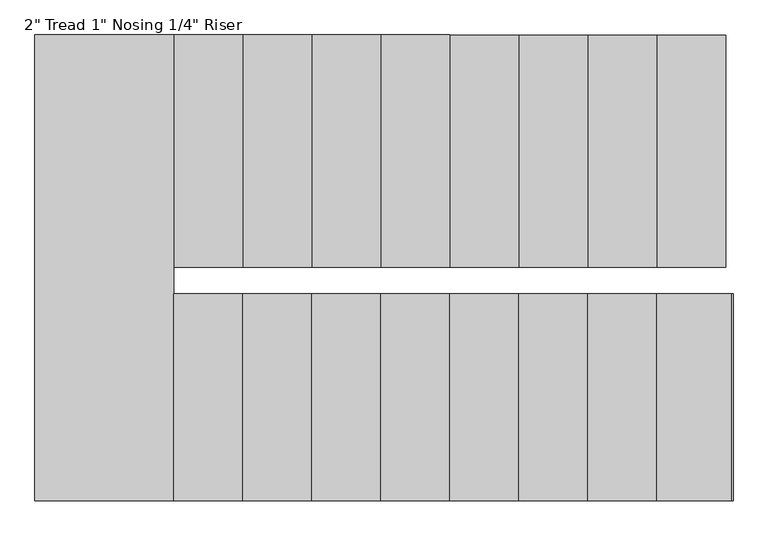
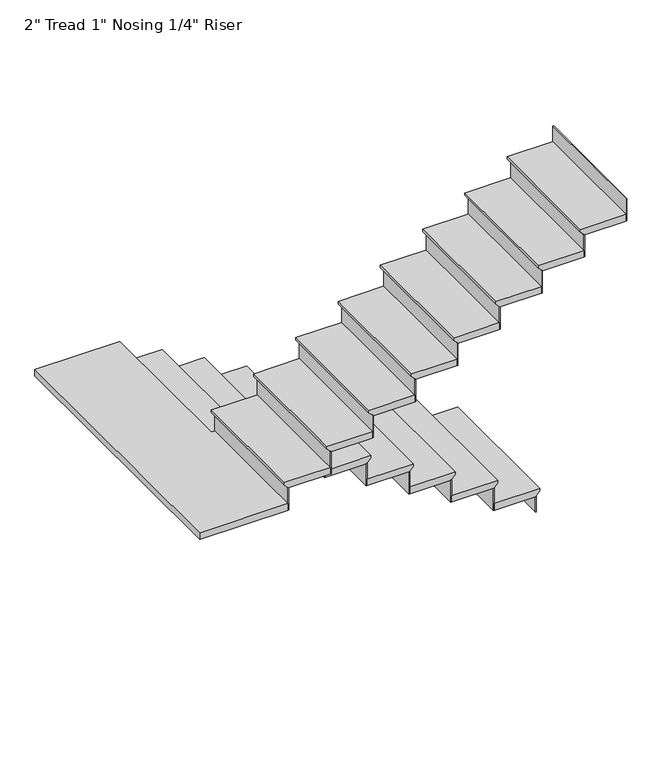
"""IFC4 building model written with IfcOpenShell, lengths in millimetres: stair flight geometry."""

from ifc_helpers import new_model, si_unit, origin, place, context, project, spatial, faceted_brep, source, transform, mapped, element, save


def stair_flight_67f7f0a7(model_context):
    return source(origin(), model_context, "Body", "Brep", [
        faceted_brep([(4295.1355783, 9969.5, 6246.2833333), (4295.1355783, 9969.5, 6265.3333333), (4295.1355783, 8944.6068332, 6265.3333333), (4295.1355783, 8944.6068332, 6246.2833333), (4269.7355783, 9969.5, 6220.8833333), (4269.7355783, 8944.6068332, 6220.8833333), (3964.9355783, 9969.5, 6265.3333333), (3964.9355783, 8944.6068332, 6265.3333333), (4269.7355783, 8944.6068332, 6214.5333333), (3964.9355783, 8944.6068332, 6214.5333333), (3964.9355783, 9969.5, 6214.5333333), (4269.7355783, 9969.5, 6214.5333333)], [[[0, 1, 2, 3]], [[4, 0, 3, 5]], [[2, 1, 6, 7]], [[8, 9, 10, 11]], [[2, 7, 9, 8, 5, 3]], [[8, 11, 4, 5]], [[6, 1, 0, 4, 11, 10]], [[7, 6, 10, 9]]]),
        faceted_brep([(4269.7355783, 9969.5, 6214.5333333), (4269.7355783, 9969.5, 6096.0), (4263.3855783, 9969.5, 6096.0), (4263.3855783, 9969.5, 6214.5333333), (4269.7355783, 8944.6068332, 6214.5333333), (4263.3855783, 8944.6068332, 6214.5333333), (4263.3855783, 8944.6068332, 6096.0), (4269.7355783, 8944.6068332, 6096.0)], [[[0, 1, 2, 3]], [[4, 5, 6, 7]], [[1, 0, 4, 7]], [[2, 1, 7, 6]], [[3, 2, 6, 5]], [[0, 3, 5, 4]]]),
        faceted_brep([(3964.9355783, 9969.5, 6383.8666667), (3964.9355783, 9969.5, 6214.5333333), (3958.5855783, 9969.5, 6214.5333333), (3958.5855783, 9969.5, 6383.8666667), (3964.9355783, 8944.6068332, 6383.8666667), (3958.5855783, 8944.6068332, 6383.8666667), (3958.5855783, 8944.6068332, 6214.5333333), (3964.9355783, 8944.6068332, 6214.5333333)], [[[0, 1, 2, 3]], [[4, 5, 6, 7]], [[1, 0, 4, 7]], [[2, 1, 7, 6]], [[3, 2, 6, 5]], [[0, 3, 5, 4]]]),
        faceted_brep([(3990.3355783, 8944.6068332, 6434.6666667), (3990.3355783, 9969.5, 6434.6666667), (3660.1355783, 9969.5, 6434.6666667), (3660.1355783, 8944.6068332, 6434.6666667), (3964.9355783, 8944.6068332, 6383.8666667), (3660.1355783, 8944.6068332, 6383.8666667), (3660.1355783, 9969.5, 6383.8666667), (3964.9355783, 9969.5, 6383.8666667), (3964.9355783, 8944.6068332, 6390.2166667), (3990.3355783, 8944.6068332, 6415.6166667), (3964.9355783, 9969.5, 6390.2166667), (3990.3355783, 9969.5, 6415.6166667)], [[[0, 1, 2, 3]], [[4, 5, 6, 7]], [[0, 3, 5, 4, 8, 9]], [[4, 7, 10, 8]], [[2, 1, 11, 10, 7, 6]], [[3, 2, 6, 5]], [[11, 1, 0, 9]], [[10, 11, 9, 8]]]),
        faceted_brep([(3660.1355783, 9969.5, 6553.2), (3660.1355783, 9969.5, 6383.8666667), (3653.7855783, 9969.5, 6383.8666667), (3653.7855783, 9969.5, 6553.2), (3660.1355783, 8944.6068332, 6553.2), (3653.7855783, 8944.6068332, 6553.2), (3653.7855783, 8944.6068332, 6383.8666667), (3660.1355783, 8944.6068332, 6383.8666667)], [[[0, 1, 2, 3]], [[4, 5, 6, 7]], [[1, 0, 4, 7]], [[2, 1, 7, 6]], [[3, 2, 6, 5]], [[0, 3, 5, 4]]]),
        faceted_brep([(3685.5355783, 8944.6068332, 6604.0), (3685.5355783, 9969.5, 6604.0), (3355.3355783, 9969.5, 6604.0), (3355.3355783, 8944.6068332, 6604.0), (3660.1355783, 8944.6068332, 6553.2), (3355.3355783, 8944.6068332, 6553.2), (3355.3355783, 9969.5, 6553.2), (3660.1355783, 9969.5, 6553.2), (3660.1355783, 8944.6068332, 6559.55), (3685.5355783, 8944.6068332, 6584.95), (3660.1355783, 9969.5, 6559.55), (3685.5355783, 9969.5, 6584.95)], [[[0, 1, 2, 3]], [[4, 5, 6, 7]], [[0, 3, 5, 4, 8, 9]], [[4, 7, 10, 8]], [[2, 1, 11, 10, 7, 6]], [[3, 2, 6, 5]], [[11, 1, 0, 9]], [[10, 11, 9, 8]]]),
        faceted_brep([(3355.3355783, 9969.5, 6722.5333333), (3355.3355783, 9969.5, 6553.2), (3348.9855783, 9969.5, 6553.2), (3348.9855783, 9969.5, 6722.5333333), (3355.3355783, 8944.6068332, 6722.5333333), (3348.9855783, 8944.6068332, 6722.5333333), (3348.9855783, 8944.6068332, 6553.2), (3355.3355783, 8944.6068332, 6553.2)], [[[0, 1, 2, 3]], [[4, 5, 6, 7]], [[1, 0, 4, 7]], [[2, 1, 7, 6]], [[3, 2, 6, 5]], [[0, 3, 5, 4]]]),
        faceted_brep([(3380.7355783, 8944.6068332, 6773.3333333), (3380.7355783, 9969.5, 6773.3333333), (3050.5355783, 9969.5, 6773.3333333), (3050.5355783, 8944.6068332, 6773.3333333), (3355.3355783, 8944.6068332, 6722.5333333), (3050.5355783, 8944.6068332, 6722.5333333), (3050.5355783, 9969.5, 6722.5333333), (3355.3355783, 9969.5, 6722.5333333), (3355.3355783, 8944.6068332, 6728.8833333), (3380.7355783, 8944.6068332, 6754.2833333), (3355.3355783, 9969.5, 6728.8833333), (3380.7355783, 9969.5, 6754.2833333)], [[[0, 1, 2, 3]], [[4, 5, 6, 7]], [[0, 3, 5, 4, 8, 9]], [[4, 7, 10, 8]], [[2, 1, 11, 10, 7, 6]], [[3, 2, 6, 5]], [[11, 1, 0, 9]], [[10, 11, 9, 8]]]),
        faceted_brep([(3050.5355783, 9969.5, 6891.8666667), (3050.5355783, 9969.5, 6722.5333333), (3044.1855783, 9969.5, 6722.5333333), (3044.1855783, 9969.5, 6891.8666667), (3050.5355783, 8944.6068332, 6891.8666667), (3044.1855783, 8944.6068332, 6891.8666667), (3044.1855783, 8944.6068332, 6722.5333333), (3050.5355783, 8944.6068332, 6722.5333333)], [[[0, 1, 2, 3]], [[4, 5, 6, 7]], [[1, 0, 4, 7]], [[2, 1, 7, 6]], [[3, 2, 6, 5]], [[0, 3, 5, 4]]]),
        faceted_brep([(3075.9355783, 8944.6068332, 6942.6666667), (3075.9355783, 9969.5, 6942.6666667), (2745.7355783, 9969.5, 6942.6666667), (2745.7355783, 8944.6068332, 6942.6666667), (3050.5355783, 8944.6068332, 6891.8666667), (2745.7355783, 8944.6068332, 6891.8666667), (2745.7355783, 9969.5, 6891.8666667), (3050.5355783, 9969.5, 6891.8666667), (3050.5355783, 8944.6068332, 6898.2166667), (3075.9355783, 8944.6068332, 6923.6166667), (3050.5355783, 9969.5, 6898.2166667), (3075.9355783, 9969.5, 6923.6166667)], [[[0, 1, 2, 3]], [[4, 5, 6, 7]], [[0, 3, 5, 4, 8, 9]], [[4, 7, 10, 8]], [[2, 1, 11, 10, 7, 6]], [[3, 2, 6, 5]], [[11, 1, 0, 9]], [[10, 11, 9, 8]]]),
        faceted_brep([(2745.7355783, 9969.5, 7061.2), (2745.7355783, 9969.5, 6891.8666667), (2739.3855783, 9969.5, 6891.8666667), (2739.3855783, 9969.5, 7061.2), (2745.7355783, 8944.6068332, 7061.2), (2739.3855783, 8944.6068332, 7061.2), (2739.3855783, 8944.6068332, 6891.8666667), (2745.7355783, 8944.6068332, 6891.8666667)], [[[0, 1, 2, 3]], [[4, 5, 6, 7]], [[1, 0, 4, 7]], [[2, 1, 7, 6]], [[3, 2, 6, 5]], [[0, 3, 5, 4]]]),
        faceted_brep([(2771.1355783, 8944.6068332, 7112.0), (2771.1355783, 9969.5, 7112.0), (2440.9355783, 9969.5, 7112.0), (2440.9355783, 8944.6068332, 7112.0), (2745.7355783, 8944.6068332, 7061.2), (2440.9355783, 8944.6068332, 7061.2), (2440.9355783, 9969.5, 7061.2), (2745.7355783, 9969.5, 7061.2), (2745.7355783, 8944.6068332, 7067.55), (2771.1355783, 8944.6068332, 7092.95), (2745.7355783, 9969.5, 7067.55), (2771.1355783, 9969.5, 7092.95)], [[[0, 1, 2, 3]], [[4, 5, 6, 7]], [[0, 3, 5, 4, 8, 9]], [[4, 7, 10, 8]], [[2, 1, 11, 10, 7, 6]], [[3, 2, 6, 5]], [[11, 1, 0, 9]], [[10, 11, 9, 8]]]),
        faceted_brep([(2440.9355783, 9969.5, 7230.5333333), (2440.9355783, 9969.5, 7061.2), (2434.5855783, 9969.5, 7061.2), (2434.5855783, 9969.5, 7230.5333333), (2440.9355783, 8944.6068332, 7230.5333333), (2434.5855783, 8944.6068332, 7230.5333333), (2434.5855783, 8944.6068332, 7061.2), (2440.9355783, 8944.6068332, 7061.2)], [[[0, 1, 2, 3]], [[4, 5, 6, 7]], [[1, 0, 4, 7]], [[2, 1, 7, 6]], [[3, 2, 6, 5]], [[0, 3, 5, 4]]]),
        faceted_brep([(2466.3355783, 8944.6068332, 7281.3333333), (2466.3355783, 9969.5, 7281.3333333), (2136.1355783, 9969.5, 7281.3333333), (2136.1355783, 8944.6068332, 7281.3333333), (2440.9355783, 8944.6068332, 7230.5333333), (2136.1355783, 8944.6068332, 7230.5333333), (2136.1355783, 9969.5, 7230.5333333), (2440.9355783, 9969.5, 7230.5333333), (2440.9355783, 8944.6068332, 7236.8833333), (2466.3355783, 8944.6068332, 7262.2833333), (2440.9355783, 9969.5, 7236.8833333), (2466.3355783, 9969.5, 7262.2833333)], [[[0, 1, 2, 3]], [[4, 5, 6, 7]], [[0, 3, 5, 4, 8, 9]], [[4, 7, 10, 8]], [[2, 1, 11, 10, 7, 6]], [[3, 2, 6, 5]], [[11, 1, 0, 9]], [[10, 11, 9, 8]]]),
        faceted_brep([(2136.1355783, 9969.5, 7399.8666667), (2136.1355783, 9969.5, 7230.5333333), (2129.7855783, 9969.5, 7230.5333333), (2129.7855783, 9969.5, 7399.8666667), (2136.1355783, 8944.6068332, 7399.8666667), (2129.7855783, 8944.6068332, 7399.8666667), (2129.7855783, 8944.6068332, 7230.5333333), (2136.1355783, 8944.6068332, 7230.5333333)], [[[0, 1, 2, 3]], [[4, 5, 6, 7]], [[1, 0, 4, 7]], [[2, 1, 7, 6]], [[3, 2, 6, 5]], [[0, 3, 5, 4]]]),
        faceted_brep([(2161.5355783, 8944.6068332, 7450.6666667), (2161.5355783, 9969.5, 7450.6666667), (1831.3355783, 9969.5, 7450.6666667), (1831.3355783, 8944.6068332, 7450.6666667), (2136.1355783, 8944.6068332, 7399.8666667), (1831.3355783, 8944.6068332, 7399.8666667), (1831.3355783, 9969.5, 7399.8666667), (2136.1355783, 9969.5, 7399.8666667), (2136.1355783, 8944.6068332, 7406.2166667), (2161.5355783, 8944.6068332, 7431.6166667), (2136.1355783, 9969.5, 7406.2166667), (2161.5355783, 9969.5, 7431.6166667)], [[[0, 1, 2, 3]], [[4, 5, 6, 7]], [[0, 3, 5, 4, 8, 9]], [[4, 7, 10, 8]], [[2, 1, 11, 10, 7, 6]], [[3, 2, 6, 5]], [[11, 1, 0, 9]], [[10, 11, 9, 8]]]),
        faceted_brep([(1831.3355783, 9969.5, 7569.2), (1831.3355783, 9969.5, 7399.8666667), (1824.9855783, 9969.5, 7399.8666667), (1824.9855783, 9969.5, 7569.2), (1831.3355783, 8944.6068332, 7569.2), (1824.9855783, 8944.6068332, 7569.2), (1824.9855783, 8944.6068332, 7399.8666667), (1831.3355783, 8944.6068332, 7399.8666667)], [[[0, 1, 2, 3]], [[4, 5, 6, 7]], [[1, 0, 4, 7]], [[2, 1, 7, 6]], [[3, 2, 6, 5]], [[0, 3, 5, 4]]]),
        faceted_brep([(1882.1355783, 8826.5, 7620.0), (1856.7355783, 8826.5, 7620.0), (1856.7355783, 9969.5, 7620.0), (1244.6, 9969.5, 7620.0), (1244.6, 7912.1, 7620.0), (1882.1355783, 7912.1, 7620.0), (1856.7355783, 8826.5, 7569.2), (1882.1355783, 8826.5, 7569.2), (1882.1355783, 7912.1, 7569.2), (1244.6, 7912.1, 7569.2), (1244.6, 9969.5, 7569.2), (1831.3355783, 9969.5, 7569.2), (1831.3355783, 8944.6068332, 7569.2), (1856.7355783, 8944.6068332, 7569.2), (1856.7355783, 8944.6068332, 7600.95), (1856.7355783, 9969.5, 7600.95), (1831.3355783, 8944.6068332, 7575.55), (1831.3355783, 9969.5, 7575.55)], [[[0, 1, 2, 3, 4, 5]], [[6, 7, 8, 9, 10, 11, 12, 13]], [[1, 0, 7, 6]], [[2, 1, 6, 13, 14, 15]], [[13, 12, 16, 14]], [[12, 11, 17, 16]], [[3, 2, 15, 17, 11, 10]], [[4, 3, 10, 9]], [[5, 4, 9, 8]], [[0, 5, 8, 7]], [[17, 15, 14, 16]]]),
        faceted_brep([(1882.1355783, 7912.1, 7738.5333333), (1882.1355783, 7912.1, 7569.2), (1888.4855783, 7912.1, 7569.2), (1888.4855783, 7912.1, 7738.5333333), (1882.1355783, 8826.5, 7738.5333333), (1888.4855783, 8826.5, 7738.5333333), (1888.4855783, 8826.5, 7569.2), (1882.1355783, 8826.5, 7569.2)], [[[0, 1, 2, 3]], [[4, 5, 6, 7]], [[1, 0, 4, 7]], [[2, 1, 7, 6]], [[3, 2, 6, 5]], [[0, 3, 5, 4]]]),
        faceted_brep([(1856.7355783, 8826.5, 7789.3333333), (1856.7355783, 7912.1, 7789.3333333), (2186.9355783, 7912.1, 7789.3333333), (2186.9355783, 8826.5, 7789.3333333), (1882.1355783, 8826.5, 7738.5333333), (2186.9355783, 8826.5, 7738.5333333), (2186.9355783, 7912.1, 7738.5333333), (1882.1355783, 7912.1, 7738.5333333), (1882.1355783, 8826.5, 7744.8833333), (1856.7355783, 8826.5, 7770.2833333), (1882.1355783, 7912.1, 7744.8833333), (1856.7355783, 7912.1, 7770.2833333)], [[[0, 1, 2, 3]], [[4, 5, 6, 7]], [[0, 3, 5, 4, 8, 9]], [[4, 7, 10, 8]], [[2, 1, 11, 10, 7, 6]], [[3, 2, 6, 5]], [[11, 1, 0, 9]], [[10, 11, 9, 8]]]),
        faceted_brep([(2186.9355783, 7912.1, 7907.8666667), (2186.9355783, 7912.1, 7738.5333333), (2193.2855783, 7912.1, 7738.5333333), (2193.2855783, 7912.1, 7907.8666667), (2186.9355783, 8826.5, 7907.8666667), (2193.2855783, 8826.5, 7907.8666667), (2193.2855783, 8826.5, 7738.5333333), (2186.9355783, 8826.5, 7738.5333333)], [[[0, 1, 2, 3]], [[4, 5, 6, 7]], [[1, 0, 4, 7]], [[2, 1, 7, 6]], [[3, 2, 6, 5]], [[0, 3, 5, 4]]]),
        faceted_brep([(2161.5355783, 8826.5, 7958.6666667), (2161.5355783, 7912.1, 7958.6666667), (2491.7355783, 7912.1, 7958.6666667), (2491.7355783, 8826.5, 7958.6666667), (2186.9355783, 8826.5, 7907.8666667), (2491.7355783, 8826.5, 7907.8666667), (2491.7355783, 7912.1, 7907.8666667), (2186.9355783, 7912.1, 7907.8666667), (2186.9355783, 8826.5, 7914.2166667), (2161.5355783, 8826.5, 7939.6166667), (2186.9355783, 7912.1, 7914.2166667), (2161.5355783, 7912.1, 7939.6166667)], [[[0, 1, 2, 3]], [[4, 5, 6, 7]], [[0, 3, 5, 4, 8, 9]], [[4, 7, 10, 8]], [[2, 1, 11, 10, 7, 6]], [[3, 2, 6, 5]], [[11, 1, 0, 9]], [[10, 11, 9, 8]]]),
        faceted_brep([(2491.7355783, 7912.1, 8077.2), (2491.7355783, 7912.1, 7907.8666667), (2498.0855783, 7912.1, 7907.8666667), (2498.0855783, 7912.1, 8077.2), (2491.7355783, 8826.5, 8077.2), (2498.0855783, 8826.5, 8077.2), (2498.0855783, 8826.5, 7907.8666667), (2491.7355783, 8826.5, 7907.8666667)], [[[0, 1, 2, 3]], [[4, 5, 6, 7]], [[1, 0, 4, 7]], [[2, 1, 7, 6]], [[3, 2, 6, 5]], [[0, 3, 5, 4]]]),
        faceted_brep([(2466.3355783, 8826.5, 8128.0), (2466.3355783, 7912.1, 8128.0), (2796.5355783, 7912.1, 8128.0), (2796.5355783, 8826.5, 8128.0), (2491.7355783, 8826.5, 8077.2), (2796.5355783, 8826.5, 8077.2), (2796.5355783, 7912.1, 8077.2), (2491.7355783, 7912.1, 8077.2), (2491.7355783, 8826.5, 8083.55), (2466.3355783, 8826.5, 8108.95), (2491.7355783, 7912.1, 8083.55), (2466.3355783, 7912.1, 8108.95)], [[[0, 1, 2, 3]], [[4, 5, 6, 7]], [[0, 3, 5, 4, 8, 9]], [[4, 7, 10, 8]], [[2, 1, 11, 10, 7, 6]], [[3, 2, 6, 5]], [[11, 1, 0, 9]], [[10, 11, 9, 8]]]),
        faceted_brep([(2796.5355783, 7912.1, 8246.5333333), (2796.5355783, 7912.1, 8077.2), (2802.8855783, 7912.1, 8077.2), (2802.8855783, 7912.1, 8246.5333333), (2796.5355783, 8826.5, 8246.5333333), (2802.8855783, 8826.5, 8246.5333333), (2802.8855783, 8826.5, 8077.2), (2796.5355783, 8826.5, 8077.2)], [[[0, 1, 2, 3]], [[4, 5, 6, 7]], [[1, 0, 4, 7]], [[2, 1, 7, 6]], [[3, 2, 6, 5]], [[0, 3, 5, 4]]]),
        faceted_brep([(2771.1355783, 8826.5, 8297.3333333), (2771.1355783, 7912.1, 8297.3333333), (3101.3355783, 7912.1, 8297.3333333), (3101.3355783, 8826.5, 8297.3333333), (2796.5355783, 8826.5, 8246.5333333), (3101.3355783, 8826.5, 8246.5333333), (3101.3355783, 7912.1, 8246.5333333), (2796.5355783, 7912.1, 8246.5333333), (2796.5355783, 8826.5, 8252.8833333), (2771.1355783, 8826.5, 8278.2833333), (2796.5355783, 7912.1, 8252.8833333), (2771.1355783, 7912.1, 8278.2833333)], [[[0, 1, 2, 3]], [[4, 5, 6, 7]], [[0, 3, 5, 4, 8, 9]], [[4, 7, 10, 8]], [[2, 1, 11, 10, 7, 6]], [[3, 2, 6, 5]], [[11, 1, 0, 9]], [[10, 11, 9, 8]]]),
        faceted_brep([(3101.3355783, 7912.1, 8415.8666667), (3101.3355783, 7912.1, 8246.5333333), (3107.6855783, 7912.1, 8246.5333333), (3107.6855783, 7912.1, 8415.8666667), (3101.3355783, 8826.5, 8415.8666667), (3107.6855783, 8826.5, 8415.8666667), (3107.6855783, 8826.5, 8246.5333333), (3101.3355783, 8826.5, 8246.5333333)], [[[0, 1, 2, 3]], [[4, 5, 6, 7]], [[1, 0, 4, 7]], [[2, 1, 7, 6]], [[3, 2, 6, 5]], [[0, 3, 5, 4]]]),
        faceted_brep([(3075.9355783, 8826.5, 8466.6666667), (3075.9355783, 7912.1, 8466.6666667), (3406.1355783, 7912.1, 8466.6666667), (3406.1355783, 8826.5, 8466.6666667), (3101.3355783, 8826.5, 8415.8666667), (3406.1355783, 8826.5, 8415.8666667), (3406.1355783, 7912.1, 8415.8666667), (3101.3355783, 7912.1, 8415.8666667), (3101.3355783, 8826.5, 8422.2166667), (3075.9355783, 8826.5, 8447.6166667), (3101.3355783, 7912.1, 8422.2166667), (3075.9355783, 7912.1, 8447.6166667)], [[[0, 1, 2, 3]], [[4, 5, 6, 7]], [[0, 3, 5, 4, 8, 9]], [[4, 7, 10, 8]], [[2, 1, 11, 10, 7, 6]], [[3, 2, 6, 5]], [[11, 1, 0, 9]], [[10, 11, 9, 8]]]),
        faceted_brep([(3406.1355783, 7912.1, 8585.2), (3406.1355783, 7912.1, 8415.8666667), (3412.4855783, 7912.1, 8415.8666667), (3412.4855783, 7912.1, 8585.2), (3406.1355783, 8826.5, 8585.2), (3412.4855783, 8826.5, 8585.2), (3412.4855783, 8826.5, 8415.8666667), (3406.1355783, 8826.5, 8415.8666667)], [[[0, 1, 2, 3]], [[4, 5, 6, 7]], [[1, 0, 4, 7]], [[2, 1, 7, 6]], [[3, 2, 6, 5]], [[0, 3, 5, 4]]]),
        faceted_brep([(3380.7355783, 8826.5, 8636.0), (3380.7355783, 7912.1, 8636.0), (3710.9355783, 7912.1, 8636.0), (3710.9355783, 8826.5, 8636.0), (3406.1355783, 8826.5, 8585.2), (3710.9355783, 8826.5, 8585.2), (3710.9355783, 7912.1, 8585.2), (3406.1355783, 7912.1, 8585.2), (3406.1355783, 8826.5, 8591.55), (3380.7355783, 8826.5, 8616.95), (3406.1355783, 7912.1, 8591.55), (3380.7355783, 7912.1, 8616.95)], [[[0, 1, 2, 3]], [[4, 5, 6, 7]], [[0, 3, 5, 4, 8, 9]], [[4, 7, 10, 8]], [[2, 1, 11, 10, 7, 6]], [[3, 2, 6, 5]], [[11, 1, 0, 9]], [[10, 11, 9, 8]]]),
        faceted_brep([(3710.9355783, 7912.1, 8754.5333333), (3710.9355783, 7912.1, 8585.2), (3717.2855783, 7912.1, 8585.2), (3717.2855783, 7912.1, 8754.5333333), (3710.9355783, 8826.5, 8754.5333333), (3717.2855783, 8826.5, 8754.5333333), (3717.2855783, 8826.5, 8585.2), (3710.9355783, 8826.5, 8585.2)], [[[0, 1, 2, 3]], [[4, 5, 6, 7]], [[1, 0, 4, 7]], [[2, 1, 7, 6]], [[3, 2, 6, 5]], [[0, 3, 5, 4]]]),
        faceted_brep([(3685.5355783, 8826.5, 8805.3333333), (3685.5355783, 7912.1, 8805.3333333), (4015.7355783, 7912.1, 8805.3333333), (4015.7355783, 8826.5, 8805.3333333), (3710.9355783, 8826.5, 8754.5333333), (4015.7355783, 8826.5, 8754.5333333), (4015.7355783, 7912.1, 8754.5333333), (3710.9355783, 7912.1, 8754.5333333), (3710.9355783, 8826.5, 8760.8833333), (3685.5355783, 8826.5, 8786.2833333), (3710.9355783, 7912.1, 8760.8833333), (3685.5355783, 7912.1, 8786.2833333)], [[[0, 1, 2, 3]], [[4, 5, 6, 7]], [[0, 3, 5, 4, 8, 9]], [[4, 7, 10, 8]], [[2, 1, 11, 10, 7, 6]], [[3, 2, 6, 5]], [[11, 1, 0, 9]], [[10, 11, 9, 8]]]),
        faceted_brep([(4015.7355783, 7912.1, 8923.8666667), (4015.7355783, 7912.1, 8754.5333333), (4022.0855783, 7912.1, 8754.5333333), (4022.0855783, 7912.1, 8923.8666667), (4015.7355783, 8826.5, 8923.8666667), (4022.0855783, 8826.5, 8923.8666667), (4022.0855783, 8826.5, 8754.5333333), (4015.7355783, 8826.5, 8754.5333333)], [[[0, 1, 2, 3]], [[4, 5, 6, 7]], [[1, 0, 4, 7]], [[2, 1, 7, 6]], [[3, 2, 6, 5]], [[0, 3, 5, 4]]]),
        faceted_brep([(4320.5355783, 7912.1, 9093.2), (4320.5355783, 7912.1, 8923.8666667), (4326.8855783, 7912.1, 8923.8666667), (4326.8855783, 7912.1, 9093.2), (4320.5355783, 8826.5, 9093.2), (4326.8855783, 8826.5, 9093.2), (4326.8855783, 8826.5, 8923.8666667), (4320.5355783, 8826.5, 8923.8666667)], [[[0, 1, 2, 3]], [[4, 5, 6, 7]], [[1, 0, 4, 7]], [[2, 1, 7, 6]], [[3, 2, 6, 5]], [[0, 3, 5, 4]]]),
        faceted_brep([(3990.3355783, 8826.5, 8974.6666667), (3990.3355783, 7912.1, 8974.6666667), (4320.5355783, 7912.1, 8974.6666667), (4320.5355783, 8826.5, 8974.6666667), (4015.7355783, 8826.5, 8923.8666667), (4320.5355783, 8826.5, 8923.8666667), (4320.5355783, 7912.1, 8923.8666667), (4015.7355783, 7912.1, 8923.8666667), (4015.7355783, 8826.5, 8930.2166667), (3990.3355783, 8826.5, 8955.6166667), (4015.7355783, 7912.1, 8930.2166667), (3990.3355783, 7912.1, 8955.6166667)], [[[0, 1, 2, 3]], [[4, 5, 6, 7]], [[0, 3, 5, 4, 8, 9]], [[4, 7, 10, 8]], [[2, 1, 11, 10, 7, 6]], [[3, 2, 6, 5]], [[11, 1, 0, 9]], [[10, 11, 9, 8]]]),
    ])


if __name__ == "__main__":
    model = new_model("IFC4")
    model_context = context("Model", 3, world=origin())
    ifc_project = project(units=[si_unit("LENGTHUNIT", "METRE", prefix="MILLI")], contexts=[model_context])
    site = spatial("IfcSite", under=ifc_project)
    building = spatial("IfcBuilding", under=site)
    placement = place(None, origin())
    stair_flight_shape = stair_flight_67f7f0a7(model_context)
    element("IfcStairFlight", 1, ObjectType="2\" Tread 1\" Nosing 1/4\" Riser", at=placement, inside=building, context=model_context, shape_type="MappedRepresentation", body=[
        mapped(stair_flight_shape, transform((0.0, 0.0, 0.0), x_axis=(1.0, 0.0, 0.0), y_axis=(0.0, 1.0, 0.0), z_axis=(0.0, 0.0, 1.0))),
    ])
    save(model, "model.ifc")
